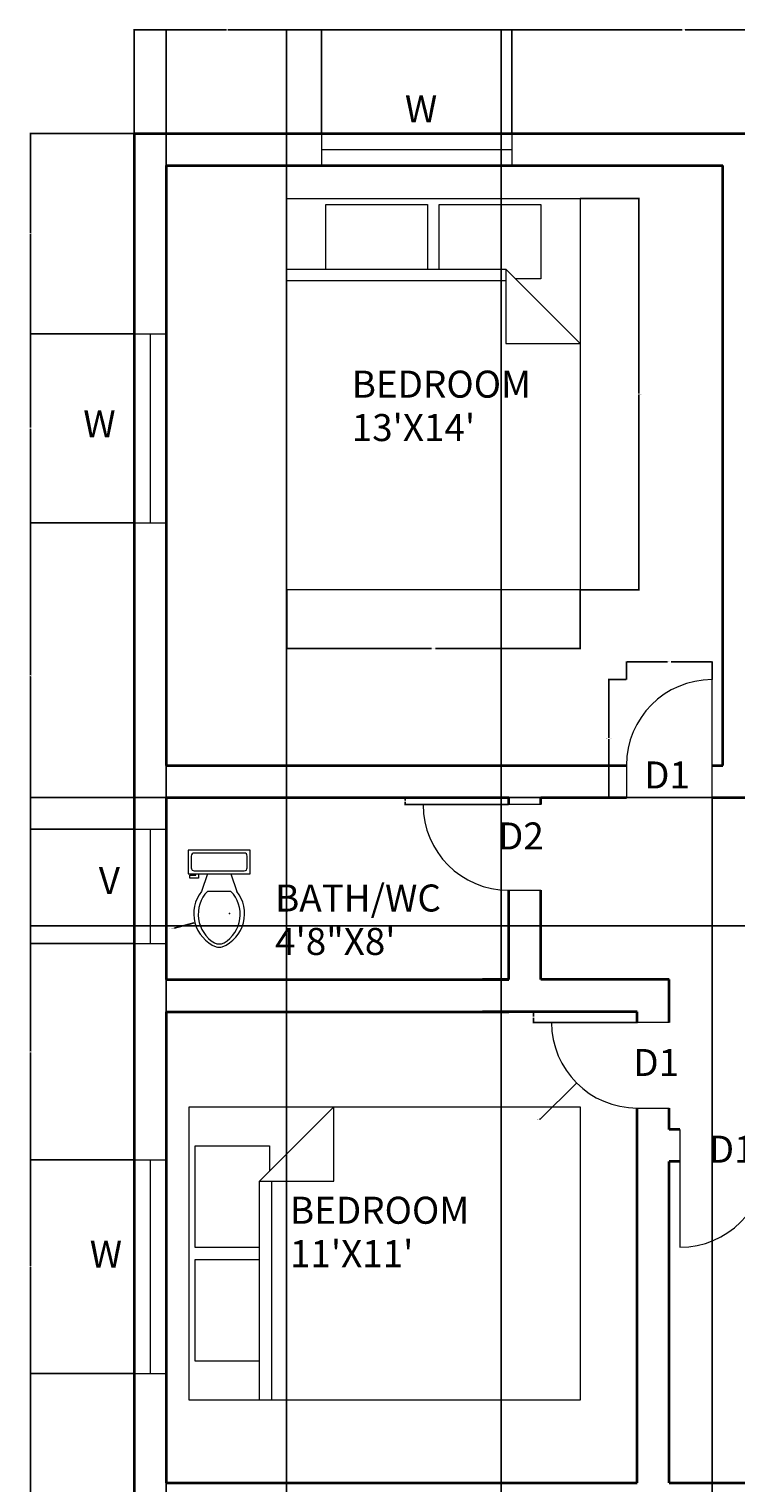
# Model space of a CAD drawing. Units: feet. Extents: x 2075 to 2525, y 1791 to 2414.
# Tile 2 of 3: x 2075 to 2273, y 2006 to 2414. Entities that reach past the tile are written whole.
import ezdxf

# ---------------------------------------------------------------- set-up
doc = ezdxf.new("R2010")
doc.units = ezdxf.units.FT
for name, color, linetype, lineweight in [('A-ANNO-DIMS', 2, 'Continuous', 18), ('A-ANNO-TEXT', 7, 'Continuous', 18), ('A-AREA-IDEN', 7, 'Continuous', 18), ('A-DOOR', 3, 'Continuous', 18), ('A-FLOR-FIXT', 8, 'Continuous', 18), ('A-FURN', 8, 'Continuous', 18), ('A-GLAZ', 4, 'Continuous', 18), ('A-WALL', 7, 'Continuous', 35)]:
    doc.layers.add(name, color=color, linetype=linetype, lineweight=lineweight)
doc.styles.get("Standard").update_dxf_attribs({"font": 'arial.ttf'})
doc.dimstyles.get("Standard").update_dxf_attribs({"dimtxt": 0.18, "dimasz": 0.18, "dimexe": 0.18, "dimexo": 0.0625, "dimgap": 0.09, "dimtad": 0, "dimtih": 1, "dimtoh": 1, "dimdec": 4, "dimzin": 0, "dimdsep": 46, "dimtxsty": 'Standard', "dimcen": 0.09, "dimadec": 0, "dimazin": 0, "dimtfac": 1, "dimtdec": 4, "dimtofl": 0, "dimtmove": 0, "dimatfit": 3, "dimfxl": 1, "dimtolj": 1, "dimtzin": 0, "dimarcsym": 0})

# ---------------------------------------------------------------- blocks, each defined once
blk = doc.blocks.new('Bed - Queen')
for p, q in [((0, -80.00003), (0, 0)), ((0, 0), (59.99999, 0)), ((59.99999, 0), (59.99999, -80.00003)), ((7.99999, -1.2), (28.79998, -1.2)), ((7.99999, -14.4), (7.99999, -1.2)), ((28.79998, -1.2), (28.79998, -14.4)), ((31.19999, -1.2), (51.99999, -1.2)), ((31.19999, -14.4), (31.19999, -1.2)), ((51.99999, -1.2), (51.99999, -16.4)), ((0, -14.4), (44.8, -14.4)), ((59.99999, -29.6), (44.8, -14.4)), ((44.8, -14.4), (44.8, -29.6)), ((44.8, -16.8), (0, -16.8)), ((51.99999, -16.4), (46.79936, -16.4)), ((44.8, -29.6), (59.99999, -29.6)), ((59.99999, -80.00003), (0, -80.00003))]:
    blk.add_line(p, q)
blk = doc.blocks.new('Toilet - top')
for p, q in [((9.5, -6), (9.5, -2)), ((-10, -8.5), (-8, -8.5)), ((-10, -9.5), (-10, -8.5)), ((-7, -9.5), (-10, -9.5)), ((-8, -8.5), (-8, -8)), ((-7, -8), (-7, -9.5)), ((-4, -8), (-6, -14)), ((4, -8), (6, -14)), ((4, -14), (-4, -14))]:
    blk.add_line(p, q)
blk.add_lwpolyline([(10.5, -8), (10.5, 0), (-10.5, 0), (-10.5, -8)], close=True)
for points in [[(-9.5, -2), (-9.5, -6)], [(8.5, -1), (-8.5, -1)], [(-8.5, -7), (8.5, -7)]]:
    blk.add_lwpolyline(points)
for centre, radius, start, end in [((-8.62, -1.88), 0.884, 81.8699, 188.1301), ((8.62, -1.88), 0.884, 351.8699, 98.1301), ((-8.62, -6.12), 0.884, 171.8699, 278.1301), ((8.62, -6.12), 0.884, 261.8699, 8.1301), ((3.52, -21.58), 12.17, 141.4691, 247.9714), ((4.2, -21.82), 11.33, 136.3677, 238.9468), ((-3.52, -21.58), 12.17, 292.0284, 38.5307), ((-4.2, -21.82), 11.33, 301.053, 43.6321), ((0, -27.88), 4, 245.7318, 294.2682), ((0, -29), 4, 254.8605, 285.1395)]:
    blk.add_arc(centre, radius, start, end)
blk = doc.blocks.new('DOOR-SINGLE-SWING')
for p, q in [((24, 0), (24, 33)), ((0, 9), (0, 0))]:
    blk.add_line(p, q)
blk.add_arc((24, 9), 24, 90, 180)
blk = doc.blocks.new('*D5')
at = {"layer": 'A-ANNO-DIMS', "color": 0, "lineweight": -2, "transparency": 16777216}
for p, q in [((2241.87, 2231.33), (2236.8, 2231.33)), ((2236.98, 2231.15), (2236.98, 2215.01)), ((2236.98, 2198.51), (2236.98, 2214.65)), ((2241.87, 2198.33), (2236.8, 2198.33))]:
    blk.add_line(p, q, dxfattribs=at)
at = {"layer": 'A-ANNO-DIMS', "color": 0, "transparency": 16777216}
for points in [[(2236.95, 2231.15), (2237.01, 2231.15), (2236.98, 2231.33)], [(2236.95, 2198.51), (2237.01, 2198.51), (2236.98, 2198.33)]]:
    blk.add_solid(points, dxfattribs=at)
at = {"layer": 'Defpoints', "color": 0, "transparency": 16777216}
for p in [(2236.98, 2231.33), (2241.93, 2231.33), (2241.93, 2198.33)]:
    blk.add_point(p, dxfattribs=at)
at = {"layer": 'A-ANNO-DIMS', "color": 0, "transparency": 16777216, "insert": (2236.98, 2214.83), "char_height": 0.18, "attachment_point": 5}
blk.add_mtext('\\A1;DOOR 33 TYP.', dxfattribs=at)
blk = doc.blocks.new('*D6')
at = {"layer": 'A-ANNO-DIMS', "color": 0, "lineweight": -2, "transparency": 16777216}
for p, q in [((2241.93, 2231.39), (2241.93, 2236.46)), ((2242.11, 2236.28), (2253.4, 2236.28)), ((2265.75, 2236.28), (2254.46, 2236.28)), ((2265.93, 2231.39), (2265.93, 2236.46))]:
    blk.add_line(p, q, dxfattribs=at)
at = {"layer": 'A-ANNO-DIMS', "color": 0, "transparency": 16777216}
for points in [[(2242.11, 2236.31), (2242.11, 2236.25), (2241.93, 2236.28)], [(2265.75, 2236.31), (2265.75, 2236.25), (2265.93, 2236.28)]]:
    blk.add_solid(points, dxfattribs=at)
at = {"layer": 'Defpoints', "color": 0, "transparency": 16777216}
for p in [(2265.93, 2236.28), (2241.93, 2231.33), (2265.93, 2231.33)]:
    blk.add_point(p, dxfattribs=at)
at = {"layer": 'A-ANNO-DIMS', "color": 0, "transparency": 16777216, "insert": (2253.93, 2236.28), "char_height": 0.18, "attachment_point": 5}
blk.add_mtext('\\A1;24 TYP.', dxfattribs=at)
blk = doc.blocks.new('*D7')
at = {"layer": 'A-ANNO-DIMS', "color": 0, "lineweight": -2, "transparency": 16777216}
for p, q in [((2229, 2366.06), (2245.55, 2366.06)), ((2245.37, 2365.88), (2245.37, 2311.45)), ((2245.37, 2256.65), (2245.37, 2311.07)), ((2229, 2256.47), (2245.55, 2256.47))]:
    blk.add_line(p, q, dxfattribs=at)
at = {"layer": 'A-ANNO-DIMS', "color": 0, "transparency": 16777216}
for points in [[(2245.34, 2365.88), (2245.4, 2365.88), (2245.37, 2366.06)], [(2245.34, 2256.65), (2245.4, 2256.65), (2245.37, 2256.47)]]:
    blk.add_solid(points, dxfattribs=at)
at = {"layer": 'Defpoints', "color": 0, "transparency": 16777216}
for p in [(2228.94, 2366.06), (2245.37, 2366.06), (2228.94, 2256.47)]:
    blk.add_point(p, dxfattribs=at)
at = {"layer": 'A-ANNO-DIMS', "color": 0, "transparency": 16777216, "insert": (2245.37, 2311.26), "char_height": 0.18, "attachment_point": 5}
blk.add_mtext('\\A1;QUEEN BED 110 TYP.', dxfattribs=at)
blk = doc.blocks.new('*D8')
at = {"layer": 'A-ANNO-DIMS', "color": 0, "lineweight": -2, "transparency": 16777216}
for p, q in [((2146.74, 2256.4), (2146.74, 2239.85)), ((2228.94, 2256.4), (2228.94, 2239.85)), ((2146.92, 2240.03), (2187.31, 2240.03)), ((2228.76, 2240.03), (2188.37, 2240.03))]:
    blk.add_line(p, q, dxfattribs=at)
at = {"layer": 'A-ANNO-DIMS', "color": 0, "transparency": 16777216}
for points in [[(2146.92, 2240.06), (2146.92, 2240), (2146.74, 2240.03)], [(2228.76, 2240.06), (2228.76, 2240), (2228.94, 2240.03)]]:
    blk.add_solid(points, dxfattribs=at)
at = {"layer": 'Defpoints', "color": 0, "transparency": 16777216}
for p in [(2146.74, 2256.47), (2228.94, 2256.47), (2228.94, 2240.03)]:
    blk.add_point(p, dxfattribs=at)
at = {"layer": 'A-ANNO-DIMS', "color": 0, "transparency": 16777216, "insert": (2187.84, 2240.03), "char_height": 0.18, "attachment_point": 5}
blk.add_mtext('\\A1;82 TYP.', dxfattribs=at)
blk = doc.blocks.new('*D19')
at = {"layer": 'A-ANNO-DIMS', "color": 0, "lineweight": -2, "transparency": 16777216}
for p, q in [((2306.87, 2198.33), (2074.7, 2198.33)), ((2074.88, 2198.15), (2074.88, 2180.51)), ((2074.88, 2162.51), (2074.88, 2180.15)), ((2306.87, 2162.33), (2074.7, 2162.33))]:
    blk.add_line(p, q, dxfattribs=at)
at = {"layer": 'A-ANNO-DIMS', "color": 0, "transparency": 16777216}
for points in [[(2074.85, 2198.15), (2074.91, 2198.15), (2074.88, 2198.33)], [(2074.85, 2162.51), (2074.91, 2162.51), (2074.88, 2162.33)]]:
    blk.add_solid(points, dxfattribs=at)
at = {"layer": 'Defpoints', "color": 0, "transparency": 16777216}
for p in [(2074.88, 2198.33), (2306.93, 2198.33), (2306.93, 2162.33)]:
    blk.add_point(p, dxfattribs=at)
at = {"layer": 'A-ANNO-DIMS', "color": 0, "transparency": 16777216, "insert": (2074.88, 2180.33), "char_height": 0.18, "attachment_point": 5}
blk.add_mtext('\\A1;36', dxfattribs=at)
blk = doc.blocks.new('*D21')
at = {"layer": 'A-ANNO-DIMS', "color": 0, "lineweight": -2, "transparency": 16777216}
for p, q in [((2103.93, 2384.39), (2103.93, 2413.56)), ((2104.11, 2413.38), (2129.85, 2413.38)), ((2156.24, 2413.38), (2130.5, 2413.38)), ((2156.42, 2384.39), (2156.42, 2413.56))]:
    blk.add_line(p, q, dxfattribs=at)
at = {"layer": 'A-ANNO-DIMS', "color": 0, "transparency": 16777216}
for points in [[(2104.11, 2413.41), (2104.11, 2413.35), (2103.93, 2413.38)], [(2156.24, 2413.41), (2156.24, 2413.35), (2156.42, 2413.38)]]:
    blk.add_solid(points, dxfattribs=at)
at = {"layer": 'Defpoints', "color": 0, "transparency": 16777216}
for p in [(2156.42, 2413.38), (2103.93, 2384.33), (2156.42, 2384.33)]:
    blk.add_point(p, dxfattribs=at)
at = {"layer": 'A-ANNO-DIMS', "color": 0, "transparency": 16777216, "insert": (2130.18, 2413.38), "char_height": 0.18, "attachment_point": 5}
blk.add_mtext('\\A1;52.5', dxfattribs=at)
blk = doc.blocks.new('*D22')
at = {"layer": 'A-ANNO-DIMS', "color": 0, "lineweight": -2, "transparency": 16777216}
for p, q in [((2156.42, 2384.39), (2156.42, 2413.56)), ((2156.6, 2413.38), (2182.71, 2413.38)), ((2209.6, 2413.38), (2183.49, 2413.38)), ((2209.78, 2384.39), (2209.78, 2413.56))]:
    blk.add_line(p, q, dxfattribs=at)
at = {"layer": 'A-ANNO-DIMS', "color": 0, "transparency": 16777216}
for points in [[(2156.6, 2413.41), (2156.6, 2413.35), (2156.42, 2413.38)], [(2209.6, 2413.41), (2209.6, 2413.35), (2209.78, 2413.38)]]:
    blk.add_solid(points, dxfattribs=at)
at = {"layer": 'Defpoints', "color": 0, "transparency": 16777216}
for p in [(2209.78, 2413.38), (2156.42, 2384.33), (2209.78, 2384.33)]:
    blk.add_point(p, dxfattribs=at)
at = {"layer": 'A-ANNO-DIMS', "color": 0, "transparency": 16777216, "insert": (2183.1, 2413.38), "char_height": 0.18, "attachment_point": 5}
blk.add_mtext('\\A1;53.35', dxfattribs=at)
blk = doc.blocks.new('*D23')
at = {"layer": 'A-ANNO-DIMS', "color": 0, "lineweight": -2, "transparency": 16777216}
for p, q in [((2209.78, 2384.39), (2209.78, 2413.56)), ((2209.96, 2413.38), (2257.59, 2413.38)), ((2306.01, 2413.38), (2258.38, 2413.38)), ((2306.19, 2384.39), (2306.19, 2413.56))]:
    blk.add_line(p, q, dxfattribs=at)
at = {"layer": 'A-ANNO-DIMS', "color": 0, "transparency": 16777216}
for points in [[(2209.96, 2413.41), (2209.96, 2413.35), (2209.78, 2413.38)], [(2306.01, 2413.41), (2306.01, 2413.35), (2306.19, 2413.38)]]:
    blk.add_solid(points, dxfattribs=at)
at = {"layer": 'Defpoints', "color": 0, "transparency": 16777216}
for p in [(2306.19, 2413.38), (2209.78, 2384.33), (2306.19, 2384.33)]:
    blk.add_point(p, dxfattribs=at)
at = {"layer": 'A-ANNO-DIMS', "color": 0, "transparency": 16777216, "insert": (2257.98, 2413.38), "char_height": 0.18, "attachment_point": 5}
blk.add_mtext('\\A1;96.42', dxfattribs=at)
blk = doc.blocks.new('*D30')
at = {"layer": 'A-ANNO-DIMS', "color": 0, "lineweight": -2, "transparency": 16777216}
for p, q in [((2103.87, 2037.01), (2074.7, 2037.01)), ((2074.88, 2036.83), (2074.88, 2001.95)), ((2074.88, 1966.69), (2074.88, 2001.58)), ((2103.87, 1966.51), (2074.7, 1966.51))]:
    blk.add_line(p, q, dxfattribs=at)
at = {"layer": 'A-ANNO-DIMS', "color": 0, "transparency": 16777216}
for points in [[(2074.85, 2036.83), (2074.91, 2036.83), (2074.88, 2037.01)], [(2074.85, 1966.69), (2074.91, 1966.69), (2074.88, 1966.51)]]:
    blk.add_solid(points, dxfattribs=at)
at = {"layer": 'Defpoints', "color": 0, "transparency": 16777216}
for p in [(2074.88, 2037.01), (2103.93, 2037.01), (2103.93, 1966.51)]:
    blk.add_point(p, dxfattribs=at)
at = {"layer": 'A-ANNO-DIMS', "color": 0, "transparency": 16777216, "insert": (2074.88, 2001.76), "char_height": 0.18, "attachment_point": 5}
blk.add_mtext('\\A1;70.5', dxfattribs=at)
blk = doc.blocks.new('*D31')
at = {"layer": 'A-ANNO-DIMS', "color": 0, "lineweight": -2, "transparency": 16777216}
for p, q in [((2103.87, 2096.79), (2074.7, 2096.79)), ((2074.88, 2096.61), (2074.88, 2067.08)), ((2074.88, 2037.19), (2074.88, 2066.72)), ((2103.87, 2037.01), (2074.7, 2037.01))]:
    blk.add_line(p, q, dxfattribs=at)
at = {"layer": 'A-ANNO-DIMS', "color": 0, "transparency": 16777216}
for points in [[(2074.85, 2096.61), (2074.91, 2096.61), (2074.88, 2096.79)], [(2074.85, 2037.19), (2074.91, 2037.19), (2074.88, 2037.01)]]:
    blk.add_solid(points, dxfattribs=at)
at = {"layer": 'Defpoints', "color": 0, "transparency": 16777216}
for p in [(2074.88, 2096.79), (2103.93, 2096.79), (2103.93, 2037.01)]:
    blk.add_point(p, dxfattribs=at)
at = {"layer": 'A-ANNO-DIMS', "color": 0, "transparency": 16777216, "insert": (2074.88, 2066.9), "char_height": 0.18, "attachment_point": 5}
blk.add_mtext('\\A1;59.77', dxfattribs=at)
blk = doc.blocks.new('*D32')
at = {"layer": 'A-ANNO-DIMS', "color": 0, "lineweight": -2, "transparency": 16777216}
for p, q in [((2103.87, 2157.39), (2074.7, 2157.39)), ((2074.88, 2157.21), (2074.88, 2127.27)), ((2074.88, 2096.97), (2074.88, 2126.91)), ((2103.87, 2096.79), (2074.7, 2096.79))]:
    blk.add_line(p, q, dxfattribs=at)
at = {"layer": 'A-ANNO-DIMS', "color": 0, "transparency": 16777216}
for points in [[(2074.85, 2157.21), (2074.91, 2157.21), (2074.88, 2157.39)], [(2074.85, 2096.97), (2074.91, 2096.97), (2074.88, 2096.79)]]:
    blk.add_solid(points, dxfattribs=at)
at = {"layer": 'Defpoints', "color": 0, "transparency": 16777216}
for p in [(2074.88, 2157.39), (2103.93, 2157.39), (2103.93, 2096.79)]:
    blk.add_point(p, dxfattribs=at)
at = {"layer": 'A-ANNO-DIMS', "color": 0, "transparency": 16777216, "insert": (2074.88, 2127.09), "char_height": 0.18, "attachment_point": 5}
blk.add_mtext('\\A1;60.6', dxfattribs=at)
blk = doc.blocks.new('*D33')
at = {"layer": 'A-ANNO-DIMS', "color": 0, "lineweight": -2, "transparency": 16777216}
for p, q in [((2103.87, 2189.46), (2074.7, 2189.46)), ((2074.88, 2189.28), (2074.88, 2173.61)), ((2074.88, 2157.57), (2074.88, 2173.24)), ((2103.87, 2157.39), (2074.7, 2157.39))]:
    blk.add_line(p, q, dxfattribs=at)
at = {"layer": 'A-ANNO-DIMS', "color": 0, "transparency": 16777216}
for points in [[(2074.85, 2189.28), (2074.91, 2189.28), (2074.88, 2189.46)], [(2074.85, 2157.57), (2074.91, 2157.57), (2074.88, 2157.39)]]:
    blk.add_solid(points, dxfattribs=at)
at = {"layer": 'Defpoints', "color": 0, "transparency": 16777216}
for p in [(2074.88, 2189.46), (2103.93, 2189.46), (2103.93, 2157.39)]:
    blk.add_point(p, dxfattribs=at)
at = {"layer": 'A-ANNO-DIMS', "color": 0, "transparency": 16777216, "insert": (2074.88, 2173.43), "char_height": 0.18, "attachment_point": 5}
blk.add_mtext('\\A1;32.066', dxfattribs=at)
blk = doc.blocks.new('*D34')
at = {"layer": 'A-ANNO-DIMS', "color": 0, "lineweight": -2, "transparency": 16777216}
for p, q in [((2103.87, 2275.3), (2074.7, 2275.3)), ((2074.88, 2275.12), (2074.88, 2232.56)), ((2074.88, 2189.64), (2074.88, 2232.2)), ((2103.87, 2189.46), (2074.7, 2189.46))]:
    blk.add_line(p, q, dxfattribs=at)
at = {"layer": 'A-ANNO-DIMS', "color": 0, "transparency": 16777216}
for points in [[(2074.85, 2275.12), (2074.91, 2275.12), (2074.88, 2275.3)], [(2074.85, 2189.64), (2074.91, 2189.64), (2074.88, 2189.46)]]:
    blk.add_solid(points, dxfattribs=at)
at = {"layer": 'Defpoints', "color": 0, "transparency": 16777216}
for p in [(2074.88, 2275.3), (2103.93, 2275.3), (2103.93, 2189.46)]:
    blk.add_point(p, dxfattribs=at)
at = {"layer": 'A-ANNO-DIMS', "color": 0, "transparency": 16777216, "insert": (2074.88, 2232.38), "char_height": 0.18, "attachment_point": 5}
blk.add_mtext('\\A1;85.84', dxfattribs=at)
blk = doc.blocks.new('*D35')
at = {"layer": 'A-ANNO-DIMS', "color": 0, "lineweight": -2, "transparency": 16777216}
for p, q in [((2103.87, 2328.19), (2074.7, 2328.19)), ((2074.88, 2328.01), (2074.88, 2301.92)), ((2074.88, 2275.48), (2074.88, 2301.56)), ((2103.87, 2275.3), (2074.7, 2275.3))]:
    blk.add_line(p, q, dxfattribs=at)
at = {"layer": 'A-ANNO-DIMS', "color": 0, "transparency": 16777216}
for points in [[(2074.85, 2328.01), (2074.91, 2328.01), (2074.88, 2328.19)], [(2074.85, 2275.48), (2074.91, 2275.48), (2074.88, 2275.3)]]:
    blk.add_solid(points, dxfattribs=at)
at = {"layer": 'Defpoints', "color": 0, "transparency": 16777216}
for p in [(2074.88, 2328.19), (2103.93, 2328.19), (2103.93, 2275.3)]:
    blk.add_point(p, dxfattribs=at)
at = {"layer": 'A-ANNO-DIMS', "color": 0, "transparency": 16777216, "insert": (2074.88, 2301.74), "char_height": 0.18, "attachment_point": 5}
blk.add_mtext('\\A1;52.89', dxfattribs=at)
blk = doc.blocks.new('*D36')
at = {"layer": 'A-ANNO-DIMS', "color": 0, "lineweight": -2, "transparency": 16777216}
for p, q in [((2103.87, 2384.33), (2074.7, 2384.33)), ((2074.88, 2384.15), (2074.88, 2356.44)), ((2074.88, 2328.37), (2074.88, 2356.08)), ((2103.87, 2328.19), (2074.7, 2328.19))]:
    blk.add_line(p, q, dxfattribs=at)
at = {"layer": 'A-ANNO-DIMS', "color": 0, "transparency": 16777216}
for points in [[(2074.85, 2384.15), (2074.91, 2384.15), (2074.88, 2384.33)], [(2074.85, 2328.37), (2074.91, 2328.37), (2074.88, 2328.19)]]:
    blk.add_solid(points, dxfattribs=at)
at = {"layer": 'Defpoints', "color": 0, "transparency": 16777216}
for p in [(2074.88, 2384.33), (2103.93, 2384.33), (2103.93, 2328.19)]:
    blk.add_point(p, dxfattribs=at)
at = {"layer": 'A-ANNO-DIMS', "color": 0, "transparency": 16777216, "insert": (2074.88, 2356.26), "char_height": 0.18, "attachment_point": 5}
blk.add_mtext('\\A1;56.15', dxfattribs=at)
blk = doc.blocks.new('*D42')
at = {"layer": 'A-ANNO-DIMS', "color": 0, "lineweight": -2, "transparency": 16777216}
for p, q in [((2112.93, 1877.39), (2112.93, 2413.56)), ((2113.11, 2413.38), (2129.33, 2413.38)), ((2146.47, 2413.38), (2130.25, 2413.38)), ((2146.65, 1877.39), (2146.65, 2413.56))]:
    blk.add_line(p, q, dxfattribs=at)
at = {"layer": 'A-ANNO-DIMS', "color": 0, "transparency": 16777216}
for points in [[(2113.11, 2413.41), (2113.11, 2413.35), (2112.93, 2413.38)], [(2146.47, 2413.41), (2146.47, 2413.35), (2146.65, 2413.38)]]:
    blk.add_solid(points, dxfattribs=at)
at = {"layer": 'Defpoints', "color": 0, "transparency": 16777216}
for p in [(2146.65, 2413.38), (2112.93, 1877.33), (2146.65, 1877.33)]:
    blk.add_point(p, dxfattribs=at)
at = {"layer": 'A-ANNO-DIMS', "color": 0, "transparency": 16777216, "insert": (2129.79, 2413.38), "char_height": 0.18, "attachment_point": 5}
blk.add_mtext('\\A1;33.725', dxfattribs=at)
blk = doc.blocks.new('*D43')
at = {"layer": 'A-ANNO-DIMS', "color": 0, "lineweight": -2, "transparency": 16777216}
for p, q in [((2146.65, 1877.39), (2146.65, 2413.56)), ((2146.83, 2413.38), (2176.43, 2413.38)), ((2206.67, 2413.38), (2177.07, 2413.38)), ((2206.85, 1877.39), (2206.85, 2413.56))]:
    blk.add_line(p, q, dxfattribs=at)
at = {"layer": 'A-ANNO-DIMS', "color": 0, "transparency": 16777216}
for points in [[(2146.83, 2413.41), (2146.83, 2413.35), (2146.65, 2413.38)], [(2206.67, 2413.41), (2206.67, 2413.35), (2206.85, 2413.38)]]:
    blk.add_solid(points, dxfattribs=at)
at = {"layer": 'Defpoints', "color": 0, "transparency": 16777216}
for p in [(2206.85, 2413.38), (2146.65, 1877.33), (2206.85, 1877.33)]:
    blk.add_point(p, dxfattribs=at)
at = {"layer": 'A-ANNO-DIMS', "color": 0, "transparency": 16777216, "insert": (2176.75, 2413.38), "char_height": 0.18, "attachment_point": 5}
blk.add_mtext('\\A1;60.2', dxfattribs=at)
blk = doc.blocks.new('*D48')
at = {"layer": 'A-ANNO-DIMS', "color": 0, "lineweight": -2, "transparency": 16777216}
for p, q in [((2265.93, 2198.27), (2265.93, 1791.1)), ((2280.93, 2198.27), (2280.93, 1791.1)), ((2266.11, 1791.28), (2273.22, 1791.28)), ((2280.75, 1791.28), (2273.64, 1791.28))]:
    blk.add_line(p, q, dxfattribs=at)
at = {"layer": 'A-ANNO-DIMS', "color": 0, "transparency": 16777216}
for points in [[(2266.11, 1791.31), (2266.11, 1791.25), (2265.93, 1791.28)], [(2280.75, 1791.31), (2280.75, 1791.25), (2280.93, 1791.28)]]:
    blk.add_solid(points, dxfattribs=at)
at = {"layer": 'Defpoints', "color": 0, "transparency": 16777216}
for p in [(2265.93, 2198.33), (2280.93, 2198.33), (2280.93, 1791.28)]:
    blk.add_point(p, dxfattribs=at)
at = {"layer": 'A-ANNO-DIMS', "color": 0, "transparency": 16777216, "insert": (2273.43, 1791.28), "char_height": 0.18, "attachment_point": 5}
blk.add_mtext('\\A1;15', dxfattribs=at)
blk = doc.blocks.new('*D50')
at = {"layer": 'A-ANNO-DIMS', "color": 0, "lineweight": -2, "transparency": 16777216}
for p, q in [((2208.87, 2198.33), (2179.7, 2198.33)), ((2208.87, 2196.33), (2179.7, 2196.33)), ((2179.88, 2198.15), (2179.88, 2197.51)), ((2179.88, 2196.51), (2179.88, 2197.15))]:
    blk.add_line(p, q, dxfattribs=at)
at = {"layer": 'A-ANNO-DIMS', "color": 0, "transparency": 16777216}
for points in [[(2179.85, 2198.15), (2179.91, 2198.15), (2179.88, 2198.33)], [(2179.85, 2196.51), (2179.91, 2196.51), (2179.88, 2196.33)]]:
    blk.add_solid(points, dxfattribs=at)
at = {"layer": 'Defpoints', "color": 0, "transparency": 16777216}
for p in [(2179.88, 2198.33), (2208.93, 2198.33), (2208.93, 2196.33)]:
    blk.add_point(p, dxfattribs=at)
at = {"layer": 'A-ANNO-DIMS', "color": 0, "transparency": 16777216, "insert": (2179.88, 2197.33), "char_height": 0.18, "attachment_point": 5}
blk.add_mtext('\\A1;2', dxfattribs=at)
blk = doc.blocks.new('*D52')
at = {"layer": 'A-ANNO-DIMS', "color": 0, "lineweight": -2, "transparency": 16777216}
for p, q in [((2244.87, 2138.33), (2215.7, 2138.33)), ((2215.88, 2138.15), (2215.88, 2137.01)), ((2244.87, 2135.33), (2215.7, 2135.33)), ((2215.88, 2135.51), (2215.88, 2136.65))]:
    blk.add_line(p, q, dxfattribs=at)
at = {"layer": 'A-ANNO-DIMS', "color": 0, "transparency": 16777216}
for points in [[(2215.85, 2138.15), (2215.91, 2138.15), (2215.88, 2138.33)], [(2215.85, 2135.51), (2215.91, 2135.51), (2215.88, 2135.33)]]:
    blk.add_solid(points, dxfattribs=at)
at = {"layer": 'Defpoints', "color": 0, "transparency": 16777216}
for p in [(2215.88, 2138.33), (2244.93, 2138.33), (2244.93, 2135.33)]:
    blk.add_point(p, dxfattribs=at)
at = {"layer": 'A-ANNO-DIMS', "color": 0, "transparency": 16777216, "insert": (2215.88, 2136.83), "char_height": 0.18, "attachment_point": 5}
blk.add_mtext('\\A1;3', dxfattribs=at)
blk = doc.blocks.new('*D54')
at = {"layer": 'A-ANNO-DIMS', "color": 0, "lineweight": -2, "transparency": 16777216}
for p, q in [((2244.84, 2135.33), (2245.02, 2135.33)), ((2244.93, 2135.24), (2244.93, 2135.42)), ((2217.77, 2108.18), (2227.83, 2118.23)), ((2217.59, 2108.18), (2217.77, 2108.18))]:
    blk.add_line(p, q, dxfattribs=at)
at = {"layer": 'A-ANNO-DIMS', "color": 0, "transparency": 16777216}
blk.add_solid([(2227.81, 2118.25), (2227.85, 2118.21), (2227.96, 2118.36)], dxfattribs=at)
at = {"layer": 'Defpoints', "color": 0, "transparency": 16777216}
for p in [(2244.93, 2135.33), (2227.96, 2118.36)]:
    blk.add_point(p, dxfattribs=at)
at = {"layer": 'A-ANNO-DIMS', "color": 0, "transparency": 16777216, "insert": (2217.1, 2108.18), "char_height": 0.18, "attachment_point": 5}
blk.add_mtext('\\A1;6X R24', dxfattribs=at)
blk = doc.blocks.new('*D55')
at = {"layer": 'A-ANNO-DIMS', "color": 0, "lineweight": -2, "transparency": 16777216}
for p, q in [((2115.17, 2161.71), (2120.82, 2163.2)), ((2130.6, 2165.79), (2130.78, 2165.79)), ((2130.69, 2165.7), (2130.69, 2165.88))]:
    blk.add_line(p, q, dxfattribs=at)
at = {"layer": 'A-ANNO-DIMS', "color": 0, "transparency": 16777216}
blk.add_solid([(2120.81, 2163.22), (2120.83, 2163.17), (2120.99, 2163.24)], dxfattribs=at)
at = {"layer": 'Defpoints', "color": 0, "transparency": 16777216}
for p in [(2120.99, 2163.24), (2130.69, 2165.79)]:
    blk.add_point(p, dxfattribs=at)
at = {"layer": 'A-ANNO-DIMS', "color": 0, "transparency": 16777216, "insert": (2114.43, 2161.71), "char_height": 0.18, "attachment_point": 5}
blk.add_mtext('\\A1;4X R10.027', dxfattribs=at)

msp = doc.modelspace()

# ---------------------------------------------------------------- linework, layer by layer
at = {"layer": 'A-GLAZ'}
for p, q in [((2156.4238, 2384.3311), (2156.4238, 2375.3311)), ((2209.7752, 2384.3311), (2209.7752, 2375.3311)), ((2156.4238, 2379.8311), (2209.7752, 2379.8311)), ((2103.9279, 2328.1853), (2112.9279, 2328.1853)), ((2108.4279, 2328.1853), (2108.4279, 2275.2951)), ((2103.9279, 2275.2951), (2112.9279, 2275.2951)), ((2103.9279, 2189.4587), (2112.9279, 2189.4587)), ((2108.4279, 2189.4587), (2108.4279, 2157.3927)), ((2103.9279, 2157.3927), (2112.9279, 2157.3927)), ((2103.9279, 2096.7881), (2112.9279, 2096.7881)), ((2108.4279, 2096.7881), (2108.4279, 2037.0134)), ((2103.9279, 2037.0134), (2112.9279, 2037.0134))]:
    msp.add_line(p, q, dxfattribs=at)
at = {"layer": 'A-WALL'}
for p, q in [((2103.9279, 2384.3311), (2268.9279, 2384.3311)), ((2103.9279, 2384.3311), (2103.9279, 1868.3311)), ((2103.9279, 2384.3311), (2421.9279, 2384.3311)), ((2103.9279, 2384.3311), (2495.9279, 2384.3311)), ((2112.9279, 2375.3311), (2268.9279, 2375.3311)), ((2112.9279, 2375.3311), (2112.9279, 2207.3311)), ((2268.9279, 2207.3311), (2268.9279, 2375.3311)), ((2112.9279, 2207.3311), (2241.9279, 2207.3311)), ((2265.9279, 2207.3311), (2268.9279, 2207.3311)), ((2103.9279, 2198.3311), (2103.9279, 2147.3311)), ((2112.9279, 2198.3311), (2208.9279, 2198.3311)), ((2112.9279, 2198.3311), (2112.9279, 2147.3311)), ((2208.9279, 2196.3311), (2208.9279, 2198.3311)), ((2217.9279, 2196.3311), (2217.9279, 2198.3311)), ((2217.9279, 2198.3311), (2241.9279, 2198.3311)), ((2265.9279, 2198.3311), (2280.9279, 2198.3311)), ((2208.9279, 2147.3311), (2208.9279, 2172.3311)), ((2217.9279, 2147.3311), (2217.9279, 2172.3311)), ((2112.9279, 2147.3311), (2160.9279, 2147.3311)), ((2160.9279, 2147.3311), (2208.9279, 2147.3311)), ((2208.9279, 2147.3311), (2201.6266, 2147.3311)), ((2253.9279, 2147.3311), (2217.9279, 2147.3311)), ((2253.9279, 2135.3311), (2253.9279, 2147.3311)), ((2103.9279, 2138.3311), (2103.9279, 1868.3311)), ((2112.9279, 2138.3311), (2160.9279, 2138.3311)), ((2112.9279, 2138.3311), (2112.9279, 2006.3311)), ((2160.9279, 2138.3311), (2208.9279, 2138.3311)), ((2244.9279, 2138.3311), (2201.6266, 2138.3311)), ((2244.9279, 2135.3311), (2244.9279, 2138.3311)), ((2244.9279, 2006.3311), (2244.9279, 2111.3311)), ((2253.9279, 2105.3311), (2253.9279, 2111.3311)), ((2256.9279, 2105.3311), (2253.9279, 2105.3311)), ((2253.9279, 2006.3311), (2253.9279, 2096.3311)), ((2256.9279, 2096.3311), (2253.9279, 2096.3311)), ((2112.9279, 2006.3311), (2244.9279, 2006.3311)), ((2253.9279, 2006.3311), (2337.9279, 2006.3311))]:
    msp.add_line(p, q, dxfattribs=at)

# ---------------------------------------------------------------- block references
at = {"layer": 'A-DOOR'}
msp.add_blockref('DOOR-SINGLE-SWING', (2241.928, 2198.331), dxfattribs=at)
for p, rotation in [((2217.9281, 2172.3312), 89.9999999999989), ((2253.9281, 2111.3312), 89.99999999999841), ((2280.9278, 2105.3313), 180)]:
    msp.add_blockref('DOOR-SINGLE-SWING', p, dxfattribs=dict(at, rotation=rotation))
at = {"layer": 'A-FLOR-FIXT', "xscale": 0.823937395848298, "yscale": 0.823937395848298, "zscale": 0.823937395848298}
msp.add_blockref('Toilet - top', (2127.7909, 2183.57), dxfattribs=at)
at = {"layer": 'A-FURN', "xscale": 1.369895756219534, "yscale": 1.369895756219534, "zscale": 1.369895756219534}
msp.add_blockref('Bed - Queen', (2146.7423, 2366.0583), dxfattribs=at)
at = {"layer": 'A-FURN', "xscale": 1.369895756219534, "yscale": 1.369895756219534, "zscale": 1.369895756219534, "rotation": 90}
msp.add_blockref('Bed - Queen', (2119.3933, 2029.5048), dxfattribs=at)

# ---------------------------------------------------------------- texts
at = {"layer": 'A-ANNO-TEXT'}
for s, height, p in [('W', 7.5694, (2179.8383, 2387.4166)), ('W', 7.5694, (2089.697, 2299.1673)), ('D1', 7.56937, (2246.8871, 2200.8448)), ('D2', 7.56937, (2205.9299, 2183.7584)), ('V', 7.5694, (2094.0394, 2171.2846)), ('D1', 7.56937, (2243.8536, 2120.3091)), ('D1', 7.56937, (2264.9976, 2096.0296)), ('W', 7.5694, (2091.5063, 2066.6485))]:
    msp.add_text(s, height=height, dxfattribs=at).set_placement(p)
at = {"layer": 'A-AREA-IDEN'}
for s, p in [('BEDROOM', (2164.9394, 2310.32)), ("13'X14'", (2164.9394, 2298.1605)), ('BATH/WC', (2143.4579, 2166.3828)), ('4\'8"X8\'', (2143.4579, 2154.2233)), ('BEDROOM', (2147.6285, 2078.924)), ("11'X11'", (2147.6285, 2066.7645))]:
    msp.add_text(s, height=7.56937, dxfattribs=at).set_placement(p)

# ---------------------------------------------------------------- dimensions: what is measured, and where the dimension line sits
at = {"layer": 'A-ANNO-DIMS'}
for base, p1, p2, override, picture, middle in [((2156.4238, 2413.3811), (2103.9279, 2384.3311), (2156.4238, 2384.3311), {"dimdec": 1, "dimlfac": 1, "dimrnd": 0, "dimzin": 0, "dimdsep": 46, "dimlunit": 2}, '*D21', (2130.1759, 2413.3811)), ((2146.6525, 2413.3811), (2112.9279, 1877.3311), (2146.6525, 1877.3311), {"dimdec": 3, "dimlfac": 1, "dimrnd": 0, "dimzin": 0, "dimdsep": 46, "dimlunit": 2}, '*D42', (2129.7902, 2413.3811)), ((2206.8484, 2413.3811), (2146.6525, 1877.3311), (2206.8484, 1877.3311), {"dimdec": 1, "dimlfac": 1, "dimrnd": 0, "dimzin": 0, "dimdsep": 46, "dimlunit": 2}, '*D43', (2176.7504, 2413.3811)), ((2209.7752, 2413.3811), (2156.4238, 2384.3311), (2209.7752, 2384.3311), {"dimdec": 2, "dimlfac": 1, "dimrnd": 0, "dimzin": 0, "dimdsep": 46, "dimlunit": 2}, '*D22', (2183.0995, 2413.3811)), ((2306.1931, 2413.3811), (2209.7752, 2384.3311), (2306.1931, 2384.3311), {"dimdec": 2, "dimlfac": 1, "dimrnd": 0, "dimzin": 0, "dimdsep": 46, "dimlunit": 2}, '*D23', (2257.9841, 2413.3811)), ((2280.9279, 1791.2811), (2265.9279, 2198.3311), (2280.9279, 2198.3311), {"dimdec": 0, "dimlfac": 1, "dimrnd": 0, "dimzin": 0, "dimdsep": 46, "dimlunit": 2}, '*D48', (2273.4279, 1791.2811))]:
    dim = msp.add_linear_dim(base=base, p1=p1, p2=p2, dimstyle='Standard', override=override, dxfattribs=at)
    dim.commit()
    dim.dimension.update_dxf_attribs({"geometry": picture, "text_midpoint": middle})
for base, p1, p2, override, picture, middle in [((2074.8779, 2384.3311), (2103.9279, 2328.1853), (2103.9279, 2384.3311), {"dimdec": 2, "dimlfac": 1, "dimrnd": 0, "dimzin": 0, "dimdsep": 46, "dimlunit": 2}, '*D36', (2074.8779, 2356.2582)), ((2074.8779, 2328.1853), (2103.9279, 2275.2951), (2103.9279, 2328.1853), {"dimdec": 2, "dimlfac": 1, "dimrnd": 0, "dimzin": 0, "dimdsep": 46, "dimlunit": 2}, '*D35', (2074.8779, 2301.7402)), ((2074.8779, 2275.2951), (2103.9279, 2189.4587), (2103.9279, 2275.2951), {"dimdec": 2, "dimlfac": 1, "dimrnd": 0, "dimzin": 0, "dimdsep": 46, "dimlunit": 2}, '*D34', (2074.8779, 2232.3769)), ((2074.8779, 2198.3311), (2306.9279, 2162.3311), (2306.9279, 2198.3311), {"dimdec": 0, "dimlfac": 1, "dimrnd": 0, "dimzin": 0, "dimdsep": 46, "dimlunit": 2}, '*D19', (2074.8779, 2180.3311)), ((2179.8779, 2198.3311), (2208.9279, 2196.3311), (2208.9279, 2198.3311), {"dimdec": 0, "dimlfac": 1, "dimrnd": 0, "dimzin": 0, "dimdsep": 46, "dimlunit": 2}, '*D50', (2179.8779, 2197.3311)), ((2074.8779, 2189.4587), (2103.9279, 2157.3927), (2103.9279, 2189.4587), {"dimdec": 3, "dimlfac": 1, "dimrnd": 0, "dimzin": 0, "dimdsep": 46, "dimlunit": 2}, '*D33', (2074.8779, 2173.4257)), ((2074.8779, 2157.3927), (2103.9279, 2096.7881), (2103.9279, 2157.3927), {"dimdec": 1, "dimlfac": 1, "dimrnd": 0, "dimzin": 0, "dimdsep": 46, "dimlunit": 2}, '*D32', (2074.8779, 2127.0904)), ((2215.8779, 2138.3311), (2244.9279, 2135.3311), (2244.9279, 2138.3311), {"dimdec": 0, "dimlfac": 1, "dimrnd": 0, "dimzin": 0, "dimdsep": 46, "dimlunit": 2}, '*D52', (2215.8779, 2136.8311)), ((2074.8779, 2096.7881), (2103.9279, 2037.0134), (2103.9279, 2096.7881), {"dimdec": 2, "dimlfac": 1, "dimrnd": 0, "dimzin": 0, "dimdsep": 46, "dimlunit": 2}, '*D31', (2074.8779, 2066.9007)), ((2074.8779, 2037.0134), (2103.9279, 1966.5149), (2103.9279, 2037.0134), {"dimdec": 1, "dimlfac": 1, "dimrnd": 0, "dimzin": 0, "dimdsep": 46, "dimlunit": 2}, '*D30', (2074.8779, 2001.7641))]:
    dim = msp.add_linear_dim(base=base, p1=p1, p2=p2, angle=90, dimstyle='Standard', override=override, dxfattribs=at)
    dim.commit()
    dim.dimension.update_dxf_attribs({"geometry": picture, "text_midpoint": middle})
for base, p1, p2, text, picture, middle in [((2245.3748, 2366.0583), (2228.9361, 2256.4666), (2228.9361, 2366.0583), 'QUEEN BED <> TYP.', '*D7', (2245.3748, 2311.2624)), ((2236.9779, 2231.3311), (2241.9279, 2198.3311), (2241.9279, 2231.3311), 'DOOR <> TYP.', '*D5', (2236.9779, 2214.8311))]:
    dim = msp.add_linear_dim(base=base, p1=p1, p2=p2, angle=90, text=text, dimstyle='Standard', override={"dimdec": 0, "dimlfac": 1, "dimrnd": 0, "dimzin": 0, "dimdsep": 46, "dimlunit": 2}, dxfattribs=at)
    dim.commit()
    dim.dimension.update_dxf_attribs({"geometry": picture, "text_midpoint": middle})
for base, p1, p2, picture, middle in [((2228.9361, 2240.0278), (2146.7423, 2256.4666), (2228.9361, 2256.4666), '*D8', (2187.8392, 2240.0278)), ((2265.9279, 2236.2811), (2241.9279, 2231.3311), (2265.9279, 2231.3311), '*D6', (2253.9279, 2236.2811))]:
    dim = msp.add_linear_dim(base=base, p1=p1, p2=p2, text='<> TYP.', dimstyle='Standard', override={"dimdec": 0, "dimlfac": 1, "dimrnd": 0, "dimzin": 0, "dimdsep": 46, "dimlunit": 2}, dxfattribs=at)
    dim.commit()
    dim.dimension.update_dxf_attribs({"geometry": picture, "text_midpoint": middle})
for center, mpoint, text, override, picture, middle in [((2130.6908, 2165.789), (2120.9934, 2163.2411), '4X <>', {"dimdec": 3, "dimlfac": 1, "dimrnd": 0, "dimzin": 0, "dimdsep": 46, "dimlunit": 2}, '*D55', (2115.175, 2161.7123)), ((2244.9279, 2135.3311), (2227.957, 2118.361), '6X <>', {"dimdec": 0, "dimlfac": 1, "dimrnd": 0, "dimzin": 0, "dimdsep": 46, "dimlunit": 2}, '*D54', (2217.0958, 2108.1789))]:
    dim = msp.add_radius_dim(center=center, mpoint=mpoint, text=text, dimstyle='Standard', override=override, dxfattribs=at)
    dim.commit()
    dim.dimension.update_dxf_attribs({"geometry": picture, "text_midpoint": middle, "dimtype": 164})

doc.saveas('drawing.dxf')
